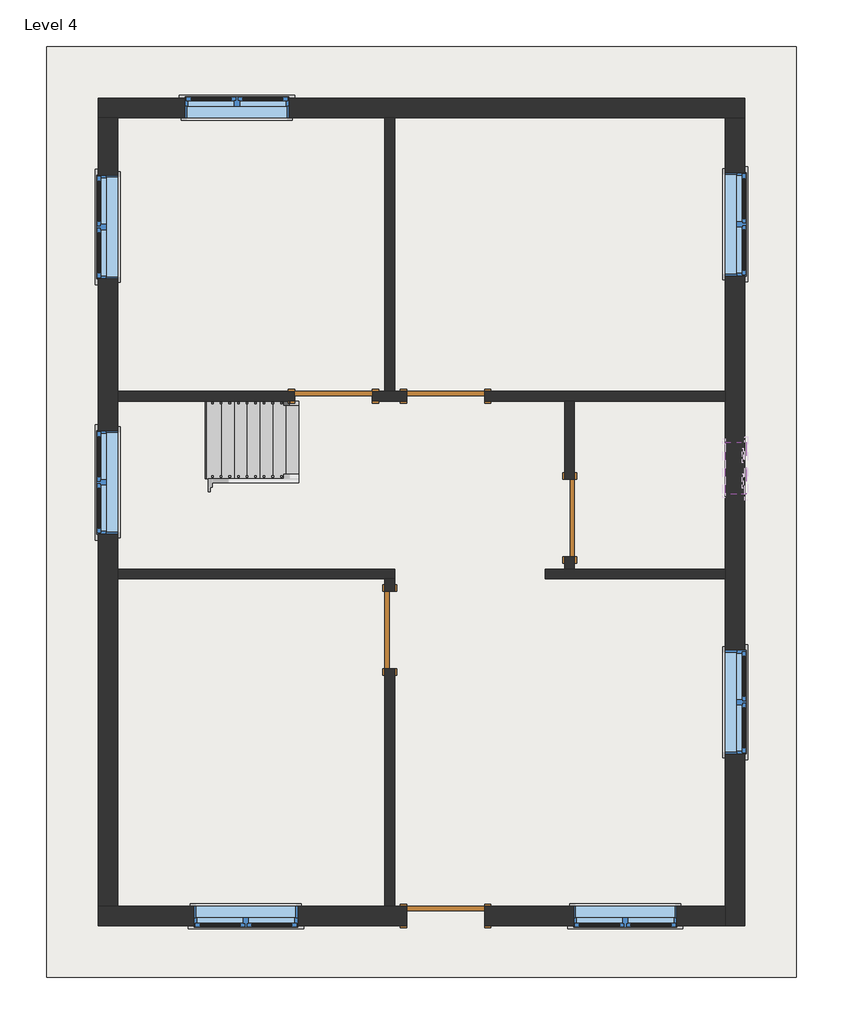
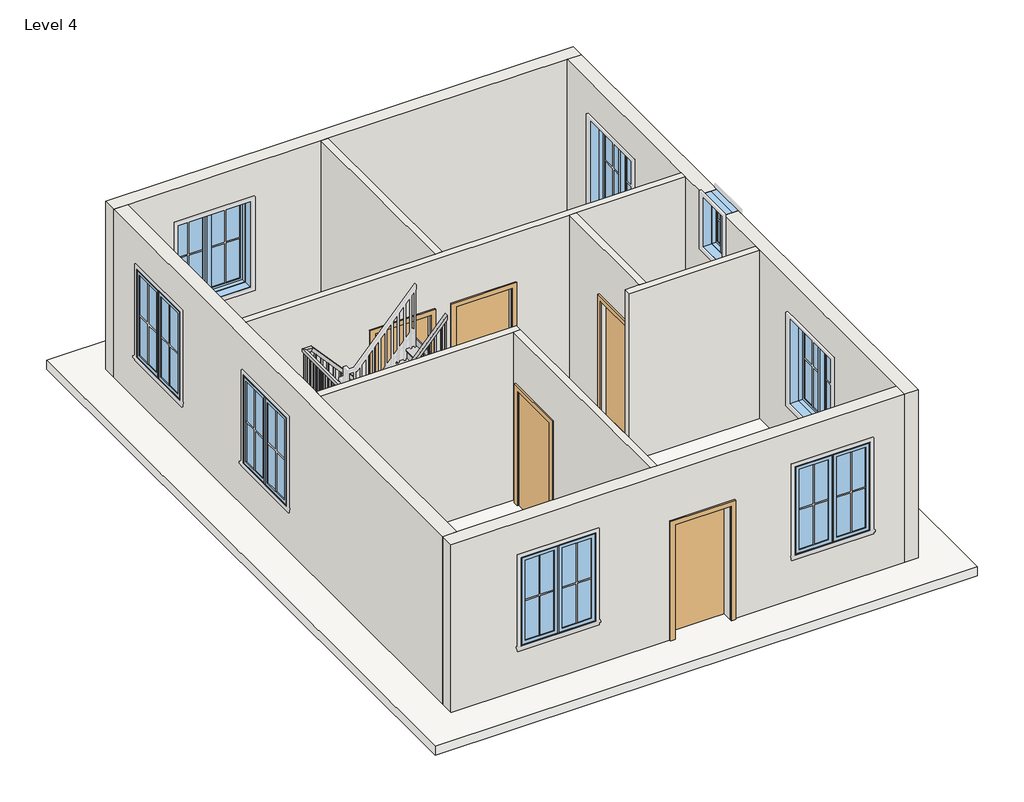
# One storey, part 1 of 2: 10 walls, 8 windows, 5 doors, 1 railing, 1 roof, 1 stair flight.
"""IFC4 building model written with IfcOpenShell, lengths in millimetres."""

from ifc_helpers import new_model, si_unit, frame, origin, place, context, project, spatial, polyline, outline, extrude, faceted_brep, transform, mapped, element, save
from components import door_e5f9f3c4, door_305aa2a5, door_a90ba1ad, stair_flight_9f5b5764, window_c417fced, window_8377141f

model = new_model("IFC4")

# Units and contexts
model_context = context("Model", 3, world=origin())
ifc_project = project(units=[si_unit("LENGTHUNIT", "METRE", prefix="MILLI")], contexts=[model_context])

# Site, building, storey
site = spatial("IfcSite", under=ifc_project)
building = spatial("IfcBuilding", under=site)
storey = spatial("IfcBuildingStorey", under=building, Name="Level 4", Elevation=9144.0)

# Doors
placement = place(None, origin())
door_shape = door_e5f9f3c4(model_context)
element("IfcDoor", 1, ObjectType="Single-Flush : 36\" x 84\"", at=placement, inside=storey, context=model_context, shape_type="MappedRepresentation", body=[
    mapped(door_shape, transform((4044.95, 10966.45, 9144.0), x_axis=(1.0, 0.0, 0.0), y_axis=(0.0, 1.0, 0.0), z_axis=(0.0, 0.0, 1.0))),
])
element("IfcDoor", 2, ObjectType="Single-Flush : 36\" x 84\"", at=placement, inside=storey, context=model_context, shape_type="MappedRepresentation", body=[
    mapped(door_shape, transform((4705.35, 8210.55, 9144.0), x_axis=(0.0, 1.0, 0.0), y_axis=(-1.0, 0.0, 0.0), z_axis=(0.0, 0.0, 1.0))),
])
element("IfcDoor", 3, ObjectType="Single-Flush : 36\" x 84\"", at=placement, inside=storey, context=model_context, shape_type="MappedRepresentation", body=[
    mapped(door_shape, transform((6826.25, 9531.35, 9144.0), x_axis=(0.0, -1.0, 0.0), y_axis=(1.0, 0.0, 0.0), z_axis=(0.0, 0.0, 1.0))),
])
door_2_shape = door_305aa2a5(model_context)
element("IfcDoor", 4, ObjectType="Single-Flush : 36\" x 84\"", at=placement, inside=storey, context=model_context, shape_type="MappedRepresentation", body=[
    mapped(door_2_shape, transform((5365.75, 10966.45, 9144.0), x_axis=(-1.0, 0.0, 0.0), y_axis=(0.0, -1.0, 0.0), z_axis=(0.0, 0.0, 1.0))),
])
door_3_shape = door_a90ba1ad(model_context)
element("IfcDoor", 5, ObjectType="Single-Flush : 36\" x 84\"", at=placement, inside=storey, context=model_context, shape_type="MappedRepresentation", body=[
    mapped(door_3_shape, transform((5365.75, 4838.7, 9144.0), x_axis=(-1.0, 0.0, 0.0), y_axis=(0.0, -1.0, 0.0), z_axis=(0.0, 0.0, 1.0))),
])

# Railing
element("IfcRailing", 6, ObjectType="Handrail - Rectangular", at=placement, inside=storey, context=model_context, shape_type="SolidModel", body=[
    faceted_brep([(3632.2, 10858.5, 10227.7333333), (3632.2, 10858.5, 10151.7950998), (3632.2, 10909.3, 10151.7950998), (3632.2, 10909.3, 10227.7333333), (2565.4, 10858.5, 11413.0666667), (2542.7755898, 10858.5, 11362.2666667), (2542.7755898, 10909.3, 11362.2666667), (2565.4, 10909.3, 11413.0666667), (2463.8, 10858.5, 11413.0666667), (2463.8, 10858.5, 11362.2666667), (2413.0, 10909.3, 11362.2666667), (2413.0, 10909.3, 11413.0666667), (2463.8, 9055.1, 11413.0666667), (2463.8, 9004.3, 11362.2666667), (2413.0, 9004.3, 11362.2666667), (2413.0, 9055.1, 11413.0666667), (2463.8, 9055.1, 11554.1777778), (2463.8, 9004.3, 11503.3777778), (2413.0, 9004.3, 11503.3777778), (2413.0, 9055.1, 11554.1777778), (2463.8, 8978.9, 11554.1777778), (2463.8, 8978.9, 11503.3777778), (2413.0, 8928.1, 11503.3777778), (2413.0, 8928.1, 11554.1777778), (2540.0, 8978.9, 11554.1777778), (2562.6244102, 8978.9, 11503.3777778), (2562.6244102, 8928.1, 11503.3777778), (2540.0, 8928.1, 11554.1777778), (3632.2, 8978.9, 12767.7333333), (3632.2, 8928.1, 12767.7333333), (3632.2, 8928.1, 12691.7950998), (3632.2, 8978.9, 12691.7950998)], [[[0, 1, 2, 3]], [[1, 0, 4, 5]], [[2, 1, 5, 6]], [[3, 2, 6, 7]], [[0, 3, 7, 4]], [[5, 4, 8, 9]], [[6, 5, 9, 10]], [[7, 6, 10, 11]], [[4, 7, 11, 8]], [[9, 8, 12, 13]], [[10, 9, 13, 14]], [[11, 10, 14, 15]], [[8, 11, 15, 12]], [[13, 12, 16, 17]], [[14, 13, 17, 18]], [[15, 14, 18, 19]], [[12, 15, 19, 16]], [[17, 16, 20, 21]], [[18, 17, 21, 22]], [[19, 18, 22, 23]], [[16, 19, 23, 20]], [[21, 20, 24, 25]], [[22, 21, 25, 26]], [[23, 22, 26, 27]], [[20, 23, 27, 24]], [[28, 29, 30, 31]], [[25, 24, 28, 31]], [[26, 25, 31, 30]], [[27, 26, 30, 29]], [[24, 27, 29, 28]]]),
    extrude(outline(polyline([(12617.7117665, 3565.525), (12596.5450998, 3546.475), (11684.0, 3546.475), (11684.0, 3565.525), (12617.7117665, 3565.525)])), frame((0.0, 8943.975, 0.0), z_axis=(0.0, 1.0, 0.0), x_axis=(0.0, 0.0, 1.0)), (0.0, 0.0, 1.0), 19.05),
    extrude(outline(polyline([(12504.8228776, 3463.925), (12483.6562109, 3444.875), (11514.6666667, 3444.875), (11514.6666667, 3463.925), (12504.8228776, 3463.925)])), frame((0.0, 8943.975, 0.0), z_axis=(0.0, 1.0, 0.0), x_axis=(0.0, 0.0, 1.0)), (0.0, 0.0, 1.0), 19.05),
    extrude(outline(polyline([(12391.9339887, 3362.325), (12370.767322, 3343.275), (11514.6666667, 3343.275), (11514.6666667, 3362.325), (12391.9339887, 3362.325)])), frame((0.0, 8943.975, 0.0), z_axis=(0.0, 1.0, 0.0), x_axis=(0.0, 0.0, 1.0)), (0.0, 0.0, 1.0), 19.05),
    extrude(outline(polyline([(12279.0450998, 3260.725), (12257.8784332, 3241.675), (11345.3333333, 3241.675), (11345.3333333, 3260.725), (12279.0450998, 3260.725)])), frame((0.0, 8943.975, 0.0), z_axis=(0.0, 1.0, 0.0), x_axis=(0.0, 0.0, 1.0)), (0.0, 0.0, 1.0), 19.05),
    extrude(outline(polyline([(12166.1562109, 3159.125), (12144.9895443, 3140.075), (11176.0, 3140.075), (11176.0, 3159.125), (12166.1562109, 3159.125)])), frame((0.0, 8943.975, 0.0), z_axis=(0.0, 1.0, 0.0), x_axis=(0.0, 0.0, 1.0)), (0.0, 0.0, 1.0), 19.05),
    extrude(outline(polyline([(12053.267322, 3057.525), (12032.1006554, 3038.475), (11176.0, 3038.475), (11176.0, 3057.525), (12053.267322, 3057.525)])), frame((0.0, 8943.975, 0.0), z_axis=(0.0, 1.0, 0.0), x_axis=(0.0, 0.0, 1.0)), (0.0, 0.0, 1.0), 19.05),
    extrude(outline(polyline([(11940.3784332, 2955.925), (11919.2117665, 2936.875), (11006.6666667, 2936.875), (11006.6666667, 2955.925), (11940.3784332, 2955.925)])), frame((0.0, 8943.975, 0.0), z_axis=(0.0, 1.0, 0.0), x_axis=(0.0, 0.0, 1.0)), (0.0, 0.0, 1.0), 19.05),
    extrude(outline(polyline([(11827.4895443, 2854.325), (11806.3228776, 2835.275), (10837.3333333, 2835.275), (10837.3333333, 2854.325), (11827.4895443, 2854.325)])), frame((0.0, 8943.975, 0.0), z_axis=(0.0, 1.0, 0.0), x_axis=(0.0, 0.0, 1.0)), (0.0, 0.0, 1.0), 19.05),
    extrude(outline(polyline([(11714.6006554, 2752.725), (11693.4339887, 2733.675), (10837.3333333, 2733.675), (10837.3333333, 2752.725), (11714.6006554, 2752.725)])), frame((0.0, 8943.975, 0.0), z_axis=(0.0, 1.0, 0.0), x_axis=(0.0, 0.0, 1.0)), (0.0, 0.0, 1.0), 19.05),
    extrude(outline(polyline([(11601.7117665, 2651.125), (11580.5450998, 2632.075), (10668.0, 2632.075), (10668.0, 2651.125), (11601.7117665, 2651.125)])), frame((0.0, 8943.975, 0.0), z_axis=(0.0, 1.0, 0.0), x_axis=(0.0, 0.0, 1.0)), (0.0, 0.0, 1.0), 19.05),
    extrude(outline(polyline([(11488.8228776, 2549.525), (11467.6562109, 2530.475), (10498.6666667, 2530.475), (10498.6666667, 2549.525), (11488.8228776, 2549.525)])), frame((0.0, 8943.975, 0.0), z_axis=(0.0, 1.0, 0.0), x_axis=(0.0, 0.0, 1.0)), (0.0, 0.0, 1.0), 19.05),
    extrude(outline(polyline([(2428.875, 9064.625), (2447.925, 9064.625), (2447.925, 9045.575), (2428.875, 9045.575), (2428.875, 9064.625)])), frame((0.0, 0.0, 10498.6666667), z_axis=(0.0, 0.0, 1.0), x_axis=(1.0, 0.0, 0.0)), (0.0, 0.0, 1.0), 863.6),
    extrude(outline(polyline([(2428.875, 9166.225), (2447.925, 9166.225), (2447.925, 9147.175), (2428.875, 9147.175), (2428.875, 9166.225)])), frame((0.0, 0.0, 10498.6666667), z_axis=(0.0, 0.0, 1.0), x_axis=(1.0, 0.0, 0.0)), (0.0, 0.0, 1.0), 863.6),
    extrude(outline(polyline([(2428.875, 9267.825), (2447.925, 9267.825), (2447.925, 9248.775), (2428.875, 9248.775), (2428.875, 9267.825)])), frame((0.0, 0.0, 10498.6666667), z_axis=(0.0, 0.0, 1.0), x_axis=(1.0, 0.0, 0.0)), (0.0, 0.0, 1.0), 863.6),
    extrude(outline(polyline([(2428.875, 9369.425), (2447.925, 9369.425), (2447.925, 9350.375), (2428.875, 9350.375), (2428.875, 9369.425)])), frame((0.0, 0.0, 10498.6666667), z_axis=(0.0, 0.0, 1.0), x_axis=(1.0, 0.0, 0.0)), (0.0, 0.0, 1.0), 863.6),
    extrude(outline(polyline([(2428.875, 9471.025), (2447.925, 9471.025), (2447.925, 9451.975), (2428.875, 9451.975), (2428.875, 9471.025)])), frame((0.0, 0.0, 10498.6666667), z_axis=(0.0, 0.0, 1.0), x_axis=(1.0, 0.0, 0.0)), (0.0, 0.0, 1.0), 863.6),
    extrude(outline(polyline([(2428.875, 9572.625), (2447.925, 9572.625), (2447.925, 9553.575), (2428.875, 9553.575), (2428.875, 9572.625)])), frame((0.0, 0.0, 10498.6666667), z_axis=(0.0, 0.0, 1.0), x_axis=(1.0, 0.0, 0.0)), (0.0, 0.0, 1.0), 863.6),
    extrude(outline(polyline([(2428.875, 9674.225), (2447.925, 9674.225), (2447.925, 9655.175), (2428.875, 9655.175), (2428.875, 9674.225)])), frame((0.0, 0.0, 10498.6666667), z_axis=(0.0, 0.0, 1.0), x_axis=(1.0, 0.0, 0.0)), (0.0, 0.0, 1.0), 863.6),
    extrude(outline(polyline([(2428.875, 9775.825), (2447.925, 9775.825), (2447.925, 9756.775), (2428.875, 9756.775), (2428.875, 9775.825)])), frame((0.0, 0.0, 10498.6666667), z_axis=(0.0, 0.0, 1.0), x_axis=(1.0, 0.0, 0.0)), (0.0, 0.0, 1.0), 863.6),
    extrude(outline(polyline([(2428.875, 9877.425), (2447.925, 9877.425), (2447.925, 9858.375), (2428.875, 9858.375), (2428.875, 9877.425)])), frame((0.0, 0.0, 10498.6666667), z_axis=(0.0, 0.0, 1.0), x_axis=(1.0, 0.0, 0.0)), (0.0, 0.0, 1.0), 863.6),
    extrude(outline(polyline([(2428.875, 9979.025), (2447.925, 9979.025), (2447.925, 9959.975), (2428.875, 9959.975), (2428.875, 9979.025)])), frame((0.0, 0.0, 10498.6666667), z_axis=(0.0, 0.0, 1.0), x_axis=(1.0, 0.0, 0.0)), (0.0, 0.0, 1.0), 863.6),
    extrude(outline(polyline([(2428.875, 10080.625), (2447.925, 10080.625), (2447.925, 10061.575), (2428.875, 10061.575), (2428.875, 10080.625)])), frame((0.0, 0.0, 10498.6666667), z_axis=(0.0, 0.0, 1.0), x_axis=(1.0, 0.0, 0.0)), (0.0, 0.0, 1.0), 863.6),
    extrude(outline(polyline([(2428.875, 10182.225), (2447.925, 10182.225), (2447.925, 10163.175), (2428.875, 10163.175), (2428.875, 10182.225)])), frame((0.0, 0.0, 10498.6666667), z_axis=(0.0, 0.0, 1.0), x_axis=(1.0, 0.0, 0.0)), (0.0, 0.0, 1.0), 863.6),
    extrude(outline(polyline([(2428.875, 10283.825), (2447.925, 10283.825), (2447.925, 10264.775), (2428.875, 10264.775), (2428.875, 10283.825)])), frame((0.0, 0.0, 10498.6666667), z_axis=(0.0, 0.0, 1.0), x_axis=(1.0, 0.0, 0.0)), (0.0, 0.0, 1.0), 863.6),
    extrude(outline(polyline([(2428.875, 10385.425), (2447.925, 10385.425), (2447.925, 10366.375), (2428.875, 10366.375), (2428.875, 10385.425)])), frame((0.0, 0.0, 10498.6666667), z_axis=(0.0, 0.0, 1.0), x_axis=(1.0, 0.0, 0.0)), (0.0, 0.0, 1.0), 863.6),
    extrude(outline(polyline([(2428.875, 10487.025), (2447.925, 10487.025), (2447.925, 10467.975), (2428.875, 10467.975), (2428.875, 10487.025)])), frame((0.0, 0.0, 10498.6666667), z_axis=(0.0, 0.0, 1.0), x_axis=(1.0, 0.0, 0.0)), (0.0, 0.0, 1.0), 863.6),
    extrude(outline(polyline([(2428.875, 10588.625), (2447.925, 10588.625), (2447.925, 10569.575), (2428.875, 10569.575), (2428.875, 10588.625)])), frame((0.0, 0.0, 10498.6666667), z_axis=(0.0, 0.0, 1.0), x_axis=(1.0, 0.0, 0.0)), (0.0, 0.0, 1.0), 863.6),
    extrude(outline(polyline([(2428.875, 10690.225), (2447.925, 10690.225), (2447.925, 10671.175), (2428.875, 10671.175), (2428.875, 10690.225)])), frame((0.0, 0.0, 10498.6666667), z_axis=(0.0, 0.0, 1.0), x_axis=(1.0, 0.0, 0.0)), (0.0, 0.0, 1.0), 863.6),
    extrude(outline(polyline([(2428.875, 10791.825), (2447.925, 10791.825), (2447.925, 10772.775), (2428.875, 10772.775), (2428.875, 10791.825)])), frame((0.0, 0.0, 10498.6666667), z_axis=(0.0, 0.0, 1.0), x_axis=(1.0, 0.0, 0.0)), (0.0, 0.0, 1.0), 863.6),
    extrude(outline(polyline([(2524.125, 10893.425), (2524.125, 10874.375), (2505.075, 10874.375), (2505.075, 10893.425), (2524.125, 10893.425)])), frame((0.0, 0.0, 10498.6666667), z_axis=(0.0, 0.0, 1.0), x_axis=(1.0, 0.0, 0.0)), (0.0, 0.0, 1.0), 863.6),
    extrude(outline(polyline([(11270.1006554, 2625.725), (11291.267322, 2606.675), (10329.3333333, 2606.675), (10329.3333333, 2625.725), (11270.1006554, 2625.725)])), frame((0.0, 10874.375, 0.0), z_axis=(0.0, 1.0, 0.0), x_axis=(0.0, 0.0, 1.0)), (0.0, 0.0, 1.0), 19.05),
    extrude(outline(polyline([(11157.2117665, 2727.325), (11178.3784332, 2708.275), (10329.3333333, 2708.275), (10329.3333333, 2727.325), (11157.2117665, 2727.325)])), frame((0.0, 10874.375, 0.0), z_axis=(0.0, 1.0, 0.0), x_axis=(0.0, 0.0, 1.0)), (0.0, 0.0, 1.0), 19.05),
    extrude(outline(polyline([(11044.3228776, 2828.925), (11065.4895443, 2809.875), (10160.0, 2809.875), (10160.0, 2828.925), (11044.3228776, 2828.925)])), frame((0.0, 10874.375, 0.0), z_axis=(0.0, 1.0, 0.0), x_axis=(0.0, 0.0, 1.0)), (0.0, 0.0, 1.0), 19.05),
    extrude(outline(polyline([(10931.4339887, 2930.525), (10952.6006554, 2911.475), (9990.6666667, 2911.475), (9990.6666667, 2930.525), (10931.4339887, 2930.525)])), frame((0.0, 10874.375, 0.0), z_axis=(0.0, 1.0, 0.0), x_axis=(0.0, 0.0, 1.0)), (0.0, 0.0, 1.0), 19.05),
    extrude(outline(polyline([(10818.5450998, 3032.125), (10839.7117665, 3013.075), (9990.6666667, 3013.075), (9990.6666667, 3032.125), (10818.5450998, 3032.125)])), frame((0.0, 10874.375, 0.0), z_axis=(0.0, 1.0, 0.0), x_axis=(0.0, 0.0, 1.0)), (0.0, 0.0, 1.0), 19.05),
    extrude(outline(polyline([(10705.6562109, 3133.725), (10726.8228776, 3114.675), (9821.3333333, 3114.675), (9821.3333333, 3133.725), (10705.6562109, 3133.725)])), frame((0.0, 10874.375, 0.0), z_axis=(0.0, 1.0, 0.0), x_axis=(0.0, 0.0, 1.0)), (0.0, 0.0, 1.0), 19.05),
    extrude(outline(polyline([(10592.767322, 3235.325), (10613.9339887, 3216.275), (9652.0, 3216.275), (9652.0, 3235.325), (10592.767322, 3235.325)])), frame((0.0, 10874.375, 0.0), z_axis=(0.0, 1.0, 0.0), x_axis=(0.0, 0.0, 1.0)), (0.0, 0.0, 1.0), 19.05),
    extrude(outline(polyline([(10479.8784332, 3336.925), (10501.0450998, 3317.875), (9652.0, 3317.875), (9652.0, 3336.925), (10479.8784332, 3336.925)])), frame((0.0, 10874.375, 0.0), z_axis=(0.0, 1.0, 0.0), x_axis=(0.0, 0.0, 1.0)), (0.0, 0.0, 1.0), 19.05),
    extrude(outline(polyline([(10366.9895443, 3438.525), (10388.1562109, 3419.475), (9482.6666667, 3419.475), (9482.6666667, 3438.525), (10366.9895443, 3438.525)])), frame((0.0, 10874.375, 0.0), z_axis=(0.0, 1.0, 0.0), x_axis=(0.0, 0.0, 1.0)), (0.0, 0.0, 1.0), 19.05),
    extrude(outline(polyline([(10254.1006554, 3540.125), (10275.267322, 3521.075), (9313.3333333, 3521.075), (9313.3333333, 3540.125), (10254.1006554, 3540.125)])), frame((0.0, 10874.375, 0.0), z_axis=(0.0, 1.0, 0.0), x_axis=(0.0, 0.0, 1.0)), (0.0, 0.0, 1.0), 19.05),
    extrude(outline(polyline([(2428.875, 8963.025), (2447.925, 8963.025), (2447.925, 8943.975), (2428.875, 8943.975), (2428.875, 8963.025)])), frame((0.0, 0.0, 10498.6666667), z_axis=(0.0, 0.0, 1.0), x_axis=(1.0, 0.0, 0.0)), (0.0, 0.0, 1.0), 1004.7111111),
    extrude(outline(polyline([(2447.925, 10893.425), (2447.925, 10874.375), (2428.875, 10874.375), (2428.875, 10893.425), (2447.925, 10893.425)])), frame((0.0, 0.0, 10498.6666667), z_axis=(0.0, 0.0, 1.0), x_axis=(1.0, 0.0, 0.0)), (0.0, 0.0, 1.0), 863.6),
    extrude(outline(polyline([(12691.7950998, 3632.2), (12670.6284332, 3613.15), (11684.0, 3613.15), (11684.0, 3632.2), (12691.7950998, 3632.2)])), frame((0.0, 8943.975, 0.0), z_axis=(0.0, 1.0, 0.0), x_axis=(0.0, 0.0, 1.0)), (0.0, 0.0, 1.0), 19.05),
    extrude(outline(polyline([(10151.7950998, 3632.2), (10172.9617665, 3613.15), (9313.3333333, 3613.15), (9313.3333333, 3632.2), (10151.7950998, 3632.2)])), frame((0.0, 10874.375, 0.0), z_axis=(0.0, 1.0, 0.0), x_axis=(0.0, 0.0, 1.0)), (0.0, 0.0, 1.0), 19.05),
])

# Roof
element("IfcRoof", 7, ObjectType="Generic - 12\"", at=placement, inside=storey, context=model_context, shape_type="SweptSolid", body=[
    extrude(outline(polyline([(660.4, 15087.6), (9499.6, 15087.6), (9499.6, 4114.8), (660.4, 4114.8), (660.4, 15087.6)])), frame((0.0, 0.0, 9144.0), z_axis=(0.0, 0.0, 1.0), x_axis=(1.0, 0.0, 0.0)), (0.0, 0.0, 1.0), 152.4),
])

# Stair flight
stair_flight_shape = stair_flight_9f5b5764(model_context)
element("IfcStairFlight", 8, ObjectType="2\" Tread 1\" Nosing 1/4\" Riser", at=placement, inside=storey, context=model_context, shape_type="MappedRepresentation", body=[
    mapped(stair_flight_shape, transform((0.0, 0.0, 0.0), x_axis=(1.0, 0.0, 0.0), y_axis=(0.0, 1.0, 0.0), z_axis=(0.0, 0.0, 1.0))),
])

# Walls
element("IfcWall", 9, ObjectType="Generic - 5\"", at=placement, inside=storey, context=model_context, shape_type="SweptSolid", body=[
    extrude(outline(polyline([(4648.2, 11023.6), (4648.2, 14249.4), (4762.5, 14249.4), (4762.5, 11023.6), (4648.2, 11023.6)])), frame((0.0, 0.0, 9144.0), z_axis=(0.0, 0.0, 1.0), x_axis=(1.0, 0.0, 0.0)), (0.0, 0.0, 1.0), 3048.0),
])
element("IfcWall", 10, ObjectType="Generic - 5\"", at=placement, inside=storey, context=model_context, shape_type="Brep", body=[
    faceted_brep([(4502.15, 10909.3, 9144.0), (4908.55, 10909.3, 9144.0), (4908.55, 10909.3, 11277.6), (5822.95, 10909.3, 11277.6), (5822.95, 10909.3, 9144.0), (6769.1, 10909.3, 9144.0), (6883.4, 10909.3, 9144.0), (8661.4, 10909.3, 9144.0), (8661.4, 10909.3, 12192.0), (6883.4, 10909.3, 12192.0), (6769.1, 10909.3, 12192.0), (1498.6, 10909.3, 12192.0), (1498.6, 10909.3, 9144.0), (3587.75, 10909.3, 9144.0), (3587.75, 10909.3, 11277.6), (4502.15, 10909.3, 11277.6), (4908.55, 11023.6, 11277.6), (4908.55, 11023.6, 9144.0), (4762.5, 11023.6, 9144.0), (4648.2, 11023.6, 9144.0), (4502.15, 11023.6, 9144.0), (4502.15, 11023.6, 11277.6), (3587.75, 11023.6, 11277.6), (3587.75, 11023.6, 9144.0), (1498.6, 11023.6, 9144.0), (1498.6, 11023.6, 12192.0), (4648.2, 11023.6, 12192.0), (4762.5, 11023.6, 12192.0), (8661.4, 11023.6, 12192.0), (8661.4, 11023.6, 9144.0), (5822.95, 11023.6, 9144.0), (5822.95, 11023.6, 11277.6)], [[[0, 1, 2, 3, 4, 5, 6, 7, 8, 9, 10, 11, 12, 13, 14, 15]], [[16, 17, 18, 19, 20, 21, 22, 23, 24, 25, 26, 27, 28, 29, 30, 31]], [[13, 12, 24, 23]], [[30, 29, 7, 6, 5, 4]], [[20, 19, 18, 17, 1, 0]], [[11, 10, 9, 8, 28, 27, 26, 25]], [[8, 7, 29, 28]], [[12, 11, 25, 24]], [[21, 20, 0, 15]], [[22, 21, 15, 14]], [[23, 22, 14, 13]], [[2, 1, 17, 16]], [[3, 2, 16, 31]], [[4, 3, 31, 30]]]),
])
element("IfcWall", 11, ObjectType="Generic - 5\"", at=placement, inside=storey, context=model_context, shape_type="SweptSolid", body=[
    extrude(outline(polyline([(9074.15, 11277.6), (9074.15, 9144.0), (8928.1, 9144.0), (8928.1, 12192.0), (10909.3, 12192.0), (10909.3, 9144.0), (9988.55, 9144.0), (9988.55, 11277.6), (9074.15, 11277.6)])), frame((6769.1, 0.0, 0.0), z_axis=(1.0, 0.0, 0.0), x_axis=(0.0, 1.0, 0.0)), (0.0, 0.0, 1.0), 114.3),
])
element("IfcWall", 12, ObjectType="Generic - 5\"", at=placement, inside=storey, context=model_context, shape_type="Brep", body=[
    faceted_brep([(1498.6, 8813.8, 9144.0), (4648.2, 8813.8, 9144.0), (4762.5, 8813.8, 9144.0), (4762.5, 8813.8, 12192.0), (4648.2, 8813.8, 12192.0), (1498.6, 8813.8, 12192.0), (1498.6, 8928.1, 9144.0), (1498.6, 8928.1, 12192.0), (4762.5, 8928.1, 12192.0), (4762.5, 8928.1, 9144.0)], [[[0, 1, 2, 3, 4, 5]], [[6, 7, 8, 9]], [[2, 1, 0, 6, 9]], [[5, 4, 3, 8, 7]], [[0, 5, 7, 6]], [[3, 2, 9, 8]]]),
])
element("IfcWall", 13, ObjectType="Generic - 5\"", at=placement, inside=storey, context=model_context, shape_type="SweptSolid", body=[
    extrude(outline(polyline([(8813.8, 9144.0), (8667.75, 9144.0), (8667.75, 11277.6), (7753.35, 11277.6), (7753.35, 9144.0), (4953.0, 9144.0), (4953.0, 12192.0), (8813.8, 12192.0), (8813.8, 9144.0)])), frame((4648.2, 0.0, 0.0), z_axis=(1.0, 0.0, 0.0), x_axis=(0.0, 1.0, 0.0)), (0.0, 0.0, 1.0), 114.3),
])
element("IfcWall", 14, ObjectType="Generic - 5\"", at=placement, inside=storey, context=model_context, shape_type="Brep", body=[
    faceted_brep([(6540.5050896, 8813.8, 9144.0), (8661.4, 8813.8, 9144.0), (8661.4, 8813.8, 12192.0), (6540.5050896, 8813.8, 12192.0), (6540.5050896, 8928.1, 9144.0), (6540.5050896, 8928.1, 12192.0), (6769.1, 8928.1, 12192.0), (6883.4, 8928.1, 12192.0), (8661.4, 8928.1, 12192.0), (8661.4, 8928.1, 9144.0), (6883.4, 8928.1, 9144.0), (6769.1, 8928.1, 9144.0)], [[[0, 1, 2, 3]], [[4, 5, 6, 7, 8, 9, 10, 11]], [[1, 0, 4, 11, 10, 9]], [[3, 2, 8, 7, 6, 5]], [[0, 3, 5, 4]], [[2, 1, 9, 8]]]),
])
element("IfcWall", 15, ObjectType="Generic - 8\"", at=placement, inside=storey, context=model_context, shape_type="Brep", body=[
    faceted_brep([(1270.0, 14249.4, 9144.0), (1498.6, 14249.4, 9144.0), (4648.2, 14249.4, 9144.0), (4762.5, 14249.4, 9144.0), (8661.4, 14249.4, 9144.0), (8890.0, 14249.4, 9144.0), (8890.0, 14249.4, 12192.0), (8661.4, 14249.4, 12192.0), (4762.5, 14249.4, 12192.0), (4648.2, 14249.4, 12192.0), (1498.6, 14249.4, 12192.0), (1270.0, 14249.4, 12192.0), (3514.725, 14249.4, 11582.4), (3514.725, 14249.4, 10058.4), (2295.525, 14249.4, 10058.4), (2295.525, 14249.4, 11582.4), (1270.0, 14478.0, 9144.0), (1270.0, 14478.0, 12192.0), (8890.0, 14478.0, 12192.0), (8890.0, 14478.0, 9144.0), (3514.725, 14478.0, 11582.4), (2295.525, 14478.0, 11582.4), (2295.525, 14478.0, 10058.4), (3514.725, 14478.0, 10058.4)], [[[0, 1, 2, 3, 4, 5, 6, 7, 8, 9, 10, 11], [12, 13, 14, 15]], [[16, 17, 18, 19], [20, 21, 22, 23]], [[5, 4, 3, 2, 1, 0, 16, 19]], [[11, 10, 9, 8, 7, 6, 18, 17]], [[6, 5, 19, 18]], [[0, 11, 17, 16]], [[13, 12, 20, 23]], [[14, 13, 23, 22]], [[15, 14, 22, 21]], [[12, 15, 21, 20]]]),
])
element("IfcWall", 16, ObjectType="Generic - 8\"", at=placement, inside=storey, context=model_context, shape_type="Brep", body=[
    faceted_brep([(8661.4, 14249.4, 9144.0), (8661.4, 11023.6, 9144.0), (8661.4, 10909.3, 9144.0), (8661.4, 8928.1, 9144.0), (8661.4, 8813.8, 9144.0), (8661.4, 4953.0, 9144.0), (8661.4, 4724.4, 9144.0), (8661.4, 4724.4, 12192.0), (8661.4, 4953.0, 12192.0), (8661.4, 8813.8, 12192.0), (8661.4, 8928.1, 12192.0), (8661.4, 9810.75, 12192.0), (8661.4, 9810.75, 11277.6), (8661.4, 10420.35, 11277.6), (8661.4, 10420.35, 12192.0), (8661.4, 10909.3, 12192.0), (8661.4, 11023.6, 12192.0), (8661.4, 14249.4, 12192.0), (8661.4, 6750.05, 11582.4), (8661.4, 6750.05, 10058.4), (8661.4, 7969.25, 10058.4), (8661.4, 7969.25, 11582.4), (8661.4, 12382.5, 11582.4), (8661.4, 12382.5, 10058.4), (8661.4, 13601.7, 10058.4), (8661.4, 13601.7, 11582.4), (8890.0, 4724.4, 9144.0), (8890.0, 14249.4, 9144.0), (8890.0, 14249.4, 12192.0), (8890.0, 10420.35, 12192.0), (8890.0, 10420.35, 11277.6), (8890.0, 9810.75, 11277.6), (8890.0, 9810.75, 12192.0), (8890.0, 4724.4, 12192.0), (8890.0, 6750.05, 10058.4), (8890.0, 6750.05, 11582.4), (8890.0, 7969.25, 11582.4), (8890.0, 7969.25, 10058.4), (8890.0, 12382.5, 10058.4), (8890.0, 12382.5, 11582.4), (8890.0, 13601.7, 11582.4), (8890.0, 13601.7, 10058.4)], [[[0, 1, 2, 3, 4, 5, 6, 7, 8, 9, 10, 11, 12, 13, 14, 15, 16, 17], [18, 19, 20, 21], [22, 23, 24, 25]], [[26, 27, 28, 29, 30, 31, 32, 33], [34, 35, 36, 37], [38, 39, 40, 41]], [[6, 5, 4, 3, 2, 1, 0, 27, 26]], [[28, 17, 16, 15, 14, 29]], [[7, 33, 32, 11, 10, 9, 8]], [[0, 17, 28, 27]], [[7, 6, 26, 33]], [[19, 18, 35, 34]], [[20, 19, 34, 37]], [[21, 20, 37, 36]], [[18, 21, 36, 35]], [[23, 22, 39, 38]], [[24, 23, 38, 41]], [[25, 24, 41, 40]], [[22, 25, 40, 39]], [[31, 12, 11, 32]], [[12, 31, 30, 13]], [[13, 30, 29, 14]]]),
])
element("IfcWall", 17, ObjectType="Generic - 8\"", at=placement, inside=storey, context=model_context, shape_type="Brep", body=[
    faceted_brep([(4908.55, 4953.0, 11277.6), (4908.55, 4953.0, 9144.0), (4762.5, 4953.0, 9144.0), (4648.2, 4953.0, 9144.0), (1498.6, 4953.0, 9144.0), (1270.0, 4953.0, 9144.0), (1270.0, 4953.0, 12192.0), (1498.6, 4953.0, 12192.0), (4648.2, 4953.0, 12192.0), (4762.5, 4953.0, 12192.0), (8661.4, 4953.0, 12192.0), (8661.4, 4953.0, 9144.0), (5822.95, 4953.0, 9144.0), (5822.95, 4953.0, 11277.6), (2400.3, 4953.0, 11582.4), (2400.3, 4953.0, 10058.4), (3619.5, 4953.0, 10058.4), (3619.5, 4953.0, 11582.4), (6872.2875, 4953.0, 11582.4), (6872.2875, 4953.0, 10058.4), (8091.4875, 4953.0, 10058.4), (8091.4875, 4953.0, 11582.4), (1270.0, 4724.4, 9144.0), (4908.55, 4724.4, 9144.0), (4908.55, 4724.4, 11277.6), (5822.95, 4724.4, 11277.6), (5822.95, 4724.4, 9144.0), (8661.4, 4724.4, 9144.0), (8661.4, 4724.4, 12192.0), (1270.0, 4724.4, 12192.0), (2400.3, 4724.4, 11582.4), (3619.5, 4724.4, 11582.4), (3619.5, 4724.4, 10058.4), (2400.3, 4724.4, 10058.4), (6872.2875, 4724.4, 11582.4), (8091.4875, 4724.4, 11582.4), (8091.4875, 4724.4, 10058.4), (6872.2875, 4724.4, 10058.4)], [[[0, 1, 2, 3, 4, 5, 6, 7, 8, 9, 10, 11, 12, 13], [14, 15, 16, 17], [18, 19, 20, 21]], [[22, 23, 24, 25, 26, 27, 28, 29], [30, 31, 32, 33], [34, 35, 36, 37]], [[12, 11, 27, 26]], [[5, 4, 3, 2, 1, 23, 22]], [[10, 9, 8, 7, 6, 29, 28]], [[11, 10, 28, 27]], [[6, 5, 22, 29]], [[24, 23, 1, 0]], [[25, 24, 0, 13]], [[26, 25, 13, 12]], [[15, 14, 30, 33]], [[16, 15, 33, 32]], [[17, 16, 32, 31]], [[14, 17, 31, 30]], [[19, 18, 34, 37]], [[20, 19, 37, 36]], [[21, 20, 36, 35]], [[18, 21, 35, 34]]]),
])
element("IfcWall", 18, ObjectType="Generic - 8\"", at=placement, inside=storey, context=model_context, shape_type="Brep", body=[
    faceted_brep([(1498.6, 4953.0, 9144.0), (1498.6, 8813.8, 9144.0), (1498.6, 8928.1, 9144.0), (1498.6, 10909.3, 9144.0), (1498.6, 11023.6, 9144.0), (1498.6, 14249.4, 9144.0), (1498.6, 14249.4, 12192.0), (1498.6, 11023.6, 12192.0), (1498.6, 10909.3, 12192.0), (1498.6, 8928.1, 12192.0), (1498.6, 8813.8, 12192.0), (1498.6, 4953.0, 12192.0), (1498.6, 13569.95, 11582.4), (1498.6, 13569.95, 10058.4), (1498.6, 12350.75, 10058.4), (1498.6, 12350.75, 11582.4), (1498.6, 10560.05, 11582.4), (1498.6, 10560.05, 10058.4), (1498.6, 9340.85, 10058.4), (1498.6, 9340.85, 11582.4), (1270.0, 14249.4, 9144.0), (1270.0, 4953.0, 9144.0), (1270.0, 4953.0, 12192.0), (1270.0, 14249.4, 12192.0), (1270.0, 13569.95, 10058.4), (1270.0, 13569.95, 11582.4), (1270.0, 12350.75, 11582.4), (1270.0, 12350.75, 10058.4), (1270.0, 10560.05, 10058.4), (1270.0, 10560.05, 11582.4), (1270.0, 9340.85, 11582.4), (1270.0, 9340.85, 10058.4)], [[[0, 1, 2, 3, 4, 5, 6, 7, 8, 9, 10, 11], [12, 13, 14, 15], [16, 17, 18, 19]], [[20, 21, 22, 23], [24, 25, 26, 27], [28, 29, 30, 31]], [[5, 4, 3, 2, 1, 0, 21, 20]], [[11, 10, 9, 8, 7, 6, 23, 22]], [[6, 5, 20, 23]], [[0, 11, 22, 21]], [[13, 12, 25, 24]], [[14, 13, 24, 27]], [[15, 14, 27, 26]], [[12, 15, 26, 25]], [[17, 16, 29, 28]], [[18, 17, 28, 31]], [[19, 18, 31, 30]], [[16, 19, 30, 29]]]),
])

# Windows
window_shape = window_c417fced(model_context)
element("IfcWindow", 19, ObjectType="Window-Casement-Double : 24\" x 36\"", at=placement, inside=storey, context=model_context, shape_type="MappedRepresentation", body=[
    mapped(window_shape, transform((8775.7, 10115.55, 10363.2), x_axis=(0.0, -1.0, 0.0), y_axis=(1.0, 0.0, 0.0), z_axis=(0.0, 0.0, 1.0))),
])
window_2_shape = window_8377141f(model_context)
element("IfcWindow", 20, ObjectType="Window-Casement-Double : 48\" x 60\"", at=placement, inside=storey, context=model_context, shape_type="MappedRepresentation", body=[
    mapped(window_2_shape, transform((7481.8875, 4838.7, 9144.0), x_axis=(-1.0, 0.0, 0.0), y_axis=(0.0, -1.0, 0.0), z_axis=(0.0, 0.0, 1.0))),
])
element("IfcWindow", 21, ObjectType="Window-Casement-Double : 48\" x 60\"", at=placement, inside=storey, context=model_context, shape_type="MappedRepresentation", body=[
    mapped(window_2_shape, transform((3009.9, 4838.7, 9144.0), x_axis=(-1.0, 0.0, 0.0), y_axis=(0.0, -1.0, 0.0), z_axis=(0.0, 0.0, 1.0))),
])
element("IfcWindow", 22, ObjectType="Window-Casement-Double : 48\" x 60\"", at=placement, inside=storey, context=model_context, shape_type="MappedRepresentation", body=[
    mapped(window_2_shape, transform((8775.7, 12992.1, 9144.0), x_axis=(0.0, -1.0, 0.0), y_axis=(1.0, 0.0, 0.0), z_axis=(0.0, 0.0, 1.0))),
])
element("IfcWindow", 23, ObjectType="Window-Casement-Double : 48\" x 60\"", at=placement, inside=storey, context=model_context, shape_type="MappedRepresentation", body=[
    mapped(window_2_shape, transform((8775.7, 7359.65, 9144.0), x_axis=(0.0, -1.0, 0.0), y_axis=(1.0, 0.0, 0.0), z_axis=(0.0, 0.0, 1.0))),
])
element("IfcWindow", 24, ObjectType="Window-Casement-Double : 48\" x 60\"", at=placement, inside=storey, context=model_context, shape_type="MappedRepresentation", body=[
    mapped(window_2_shape, transform((1384.3, 12960.35, 9144.0), x_axis=(0.0, 1.0, 0.0), y_axis=(-1.0, 0.0, 0.0), z_axis=(0.0, 0.0, 1.0))),
])
element("IfcWindow", 25, ObjectType="Window-Casement-Double : 48\" x 60\"", at=placement, inside=storey, context=model_context, shape_type="MappedRepresentation", body=[
    mapped(window_2_shape, transform((1384.3, 9950.45, 9144.0), x_axis=(0.0, 1.0, 0.0), y_axis=(-1.0, 0.0, 0.0), z_axis=(0.0, 0.0, 1.0))),
])
element("IfcWindow", 26, ObjectType="Window-Casement-Double : 48\" x 60\"", at=placement, inside=storey, context=model_context, shape_type="MappedRepresentation", body=[
    mapped(window_2_shape, transform((2905.125, 14363.7, 9144.0), x_axis=(1.0, 0.0, 0.0), y_axis=(0.0, 1.0, 0.0), z_axis=(0.0, 0.0, 1.0))),
])

save(model, "model.ifc")

# Revit data of these elements
# Type "Single-Flush : 36\" x 84\""
#   Type Mark = "1"
#   Construction Type Id = "MDOOR"
#   Assembly Code = "C1020"
#   Analytic Construction = "Metal"
#   Thickness = 0' - 2"
#   Heat Transfer Coefficient (U) = 0.651978 BTU/(h·ft²·°F)
#   Height = 7' - 0"
#   Trim Projection Ext = 0' - 1"
#   Trim Projection Int = 0' - 1"
#   Trim Width = 0' - 3"
#   Width = 3' - 0"
#   Define Thermal Properties by = 1
#   Define Thermal Properties by = 1
#   Door Material = Door - Panel
#   Frame Material = Door - Frame
#   Visual Light Transmittance = 0
#   Solar Heat Gain Coefficient = 0
#   Function = (empty or 0)
#   Wall Closure = (empty or 0)
# Type "Handrail - Rectangular"
#   Assembly Code = "C2010400"
#   built-in parameter 1008612 = 0.0416667 (stored number, unit not read)
#   built-in parameter 1008611 = 0.0416667 (stored number, unit not read)
#   built-in parameter 1008609 = 0.333333 (stored number, unit not read)
#   built-in parameter 1008604 = 0.166667 (stored number, unit not read)
#   built-in parameter 1008603 = 0.166667 (stored number, unit not read)
#   Railing Height = 3' - 0"
#   built-in parameter 1008630 = 2
#   built-in parameter 1008610 = 2
#   built-in parameter 1008618 = Baluster - Square : 3/4"
# Type "Generic - 12\""
#   Assembly Code = "B1020"
#   Layers, outside or top first: 0' - 6" no material (function 1)
# Type "Generic - 5\""
#   Assembly Code = "B2010"
#   Layers, outside or top first: 0' - 4 1/2" no material (function 1)
# Type "Generic - 8\""
#   Assembly Code = "B2010"
#   Layers, outside or top first: 0' - 9" "Parking Stripe" (function 1)
# Type "Window-Casement-Double : 24\" x 36\""
#   Type Mark = "14"
#   Fire Rating = "0.5h"
#   Assembly Code = "B2020100"
#   Analytic Construction = "Double glazing - domestic"
#   Frame Extension [instance default] = 0' - 0 1/4"
#   Window Inset [instance default] = 0' - 0"
#   Wall Thickness [instance default] = 0' - 6"
#   Interior Wall Closure [instance default] = 0' - 2 1/4"
#   Half Width = 1' - 0"
#   Visual Light Transmittance = 0.81
#   Thermal Resistance (R) = 1.8146 (h·ft²·°F)/BTU
#   Solar Heat Gain Coefficient = 0.76
#   Rough Width = 2' - 0 1/2"
#   Rough Height = 3' - 0 1/2"
#   Height = 3' - 0"
#   Heat Transfer Coefficient (U) = 0.5511 BTU/(h·ft²·°F)
#   Exterior Wall Closure [instance default] = 0' - 1 1/4"
#   Extension Jamb [instance default] = 0' - 2 1/4"
#   Default Sill Height = 3' - 0"
#   Width = 2' - 0"
#   Define Thermal Properties by = 0
#   Muntin Visibility = yes
#   Interior Trim Visibility [instance default] = yes
#   Exterior Trim Visibility [instance default] = yes
#   Extension Jamb Visibility [instance default] = yes
#   Interior Trim Material = Wood - Stained
#   Muntin Pattern = Muntin Pattern_2x2 : Muntin Pattern_2x2
#   Interior Trim = Trim-Window-Interior-Flat : Picture Frame
#   Interior Frame Material = Wood - Stained
#   Glass Panel Material = Glass
#   Exterior Trim Material = Clad - White
#   Exterior Trim = Trim-Window-Exterior-Flat : with Sill
#   Exterior Frame Material = Clad - White
#   Wall Closure = (empty or 0)
# Type "Window-Casement-Double : 48\" x 60\""
#   Type Mark = "17"
#   Fire Rating = "0.5h"
#   Assembly Code = "B2020100"
#   Analytic Construction = "Double glazing - domestic"
#   Frame Extension [instance default] = 0' - 0 1/4"
#   Window Inset [instance default] = 0' - 0"
#   Wall Thickness [instance default] = 0' - 6"
#   Interior Wall Closure [instance default] = 0' - 2 1/4"
#   Half Width = 2' - 0"
#   Visual Light Transmittance = 0.81
#   Thermal Resistance (R) = 1.8146 (h·ft²·°F)/BTU
#   Solar Heat Gain Coefficient = 0.76
#   Rough Width = 4' - 0 1/2"
#   Rough Height = 5' - 0 1/2"
#   Height = 5' - 0"
#   Heat Transfer Coefficient (U) = 0.5511 BTU/(h·ft²·°F)
#   Exterior Wall Closure [instance default] = 0' - 1 1/4"
#   Extension Jamb [instance default] = 0' - 2 1/4"
#   Default Sill Height = 3' - 0"
#   Width = 4' - 0"
#   Define Thermal Properties by = 0
#   Muntin Visibility = yes
#   Interior Trim Visibility [instance default] = yes
#   Exterior Trim Visibility [instance default] = yes
#   Extension Jamb Visibility [instance default] = yes
#   Interior Trim Material = Wood - Stained
#   Muntin Pattern = Muntin Pattern_2x2 : Muntin Pattern_2x2
#   Interior Trim = Trim-Window-Interior-Flat : Picture Frame
#   Interior Frame Material = Wood - Stained
#   Glass Panel Material = Glass
#   Exterior Trim Material = Clad - White
#   Exterior Trim = Trim-Window-Exterior-Flat : with Sill
#   Exterior Frame Material = Clad - White
#   Wall Closure = (empty or 0)
# Elements 1, 2, 3, 4, 5 (IfcDoor, "Single-Flush : 36\" x 84\"")
#   Phase Created = New Construction
#   Materials on its faces: "Door - Frame", "Door - Panel"
# Element 6 (IfcRailing, "Handrail - Rectangular")
#   Phase Created = New Construction
# Element 7 (IfcRoof, "Generic - 12\"")
#   built-in parameter 1001705 = 30.5 (stored number, unit not read)
#   built-in parameter 1001710 = 33615
#   Phase Created = New Construction
#   Materials on its faces: "Textile - Linen, Smooth", "Default Roof"
# Element 8 (IfcStairFlight, "2\" Tread 1\" Nosing 1/4\" Riser")
#   Phase Created = New Construction
# Elements 9, 10, 11, 12, 13, 14 (IfcWall, "Generic - 5\"")
#   Top Offset = 0' - 0"
#   Base Offset = 0' - 0"
#   wall height = 10' - 0"
#   Phase Created = New Construction
#   Base Constraint = Level 4
#   Top Constraint = Level 5
#   Materials on its faces: "Default Wall"
# Elements 15, 16, 17, 18 (IfcWall, "Generic - 8\"")
#   Top Offset = 0' - 0"
#   Base Offset = 0' - 0"
#   Unconnected Height = 10' - 0"
#   wall height = 10' - 0"
#   Phase Created = New Construction
#   Base Constraint = Level 4
#   Materials on its faces: "Parking Stripe", "Wood Planks"
# Element 19 (IfcWindow, "Window-Casement-Double : 24\" x 36\"")
#   Mark = "27"
#   Window Inset = 0' - 0"
#   Interior Wall Closure = 0' - 2 1/4"
#   Frame Extension = 0' - 0 1/4"
#   Exterior Wall Closure = 0' - 1 1/4"
#   Interior Trim Visibility = yes
#   Exterior Trim Visibility = yes
#   Phase Created = New Construction
#   Materials on its faces: "Wood - Stained", "Glass", "Clad - White"
# Element 20 (IfcWindow, "Window-Casement-Double : 48\" x 60\"")
#   Mark = "13"
#   Window Inset = 0' - 0"
#   Interior Wall Closure = 0' - 2 1/4"
#   Frame Extension = 0' - 0 1/4"
#   Exterior Wall Closure = 0' - 1 1/4"
#   Interior Trim Visibility = yes
#   Exterior Trim Visibility = yes
#   Phase Created = New Construction
#   Materials on its faces: "Wood - Stained", "Glass", "Clad - White"
# Element 21 (IfcWindow, "Window-Casement-Double : 48\" x 60\"")
#   Mark = "14"
#   Window Inset = 0' - 0"
#   Interior Wall Closure = 0' - 2 1/4"
#   Frame Extension = 0' - 0 1/4"
#   Exterior Wall Closure = 0' - 1 1/4"
#   Interior Trim Visibility = yes
#   Exterior Trim Visibility = yes
#   Phase Created = New Construction
#   Materials on its faces: "Wood - Stained", "Glass", "Clad - White"
# Element 22 (IfcWindow, "Window-Casement-Double : 48\" x 60\"")
#   Mark = "25"
#   Window Inset = 0' - 0"
#   Interior Wall Closure = 0' - 2 1/4"
#   Frame Extension = 0' - 0 1/4"
#   Exterior Wall Closure = 0' - 1 1/4"
#   Interior Trim Visibility = yes
#   Exterior Trim Visibility = yes
#   Phase Created = New Construction
#   Materials on its faces: "Wood - Stained", "Glass", "Clad - White"
# Element 23 (IfcWindow, "Window-Casement-Double : 48\" x 60\"")
#   Mark = "26"
#   Window Inset = 0' - 0"
#   Interior Wall Closure = 0' - 2 1/4"
#   Frame Extension = 0' - 0 1/4"
#   Exterior Wall Closure = 0' - 1 1/4"
#   Interior Trim Visibility = yes
#   Exterior Trim Visibility = yes
#   Phase Created = New Construction
#   Materials on its faces: "Wood - Stained", "Glass", "Clad - White"
# Element 24 (IfcWindow, "Window-Casement-Double : 48\" x 60\"")
#   Mark = "36"
#   Window Inset = 0' - 0"
#   Interior Wall Closure = 0' - 2 1/4"
#   Frame Extension = 0' - 0 1/4"
#   Exterior Wall Closure = 0' - 1 1/4"
#   Interior Trim Visibility = yes
#   Exterior Trim Visibility = yes
#   Phase Created = New Construction
#   Materials on its faces: "Wood - Stained", "Glass", "Clad - White"
# Element 25 (IfcWindow, "Window-Casement-Double : 48\" x 60\"")
#   Mark = "40"
#   Window Inset = 0' - 0"
#   Interior Wall Closure = 0' - 2 1/4"
#   Frame Extension = 0' - 0 1/4"
#   Exterior Wall Closure = 0' - 1 1/4"
#   Interior Trim Visibility = yes
#   Exterior Trim Visibility = yes
#   Phase Created = New Construction
#   Materials on its faces: "Wood - Stained", "Glass", "Clad - White"
# Element 26 (IfcWindow, "Window-Casement-Double : 48\" x 60\"")
#   Mark = "50"
#   Window Inset = 0' - 0"
#   Interior Wall Closure = 0' - 2 1/4"
#   Frame Extension = 0' - 0 1/4"
#   Exterior Wall Closure = 0' - 1 1/4"
#   Interior Trim Visibility = yes
#   Exterior Trim Visibility = yes
#   Phase Created = New Construction
#   Materials on its faces: "Wood - Stained", "Glass", "Clad - White"
# Materials
#   "Door - Panel": class "Wood", colour RGB 210 159 95, transparency 0, Cost = 0
#   "Door - Frame": colour RGB 118 70 51, transparency 0, Cost = 0
#   "Parking Stripe": class "Paint", colour RGB 250 250 91, transparency 0, Cost = 0
#   "Wood - Stained": class "Wood", colour RGB 224 178 126, transparency 0, Cost = 0
#   "Glass": class "Glass", colour RGB 0 128 192, transparency 0.75, Description = "Soda Lime Glass", Cost = 0
#   "Clad - White": class "Wood", colour RGB 242 242 238, transparency 0, Cost = 0
#   "Textile - Linen, Smooth": colour RGB 249 239 230, transparency 0
#   "Default Roof": colour RGB 88 101 114, transparency 0, Cost = 0
#   "Default Wall": colour RGB 128 128 128, transparency 0, Cost = 0
#   "Wood Planks": class "Wood", colour RGB 193 160 115, transparency 0, Description = "Physical material.", Cost = 0
